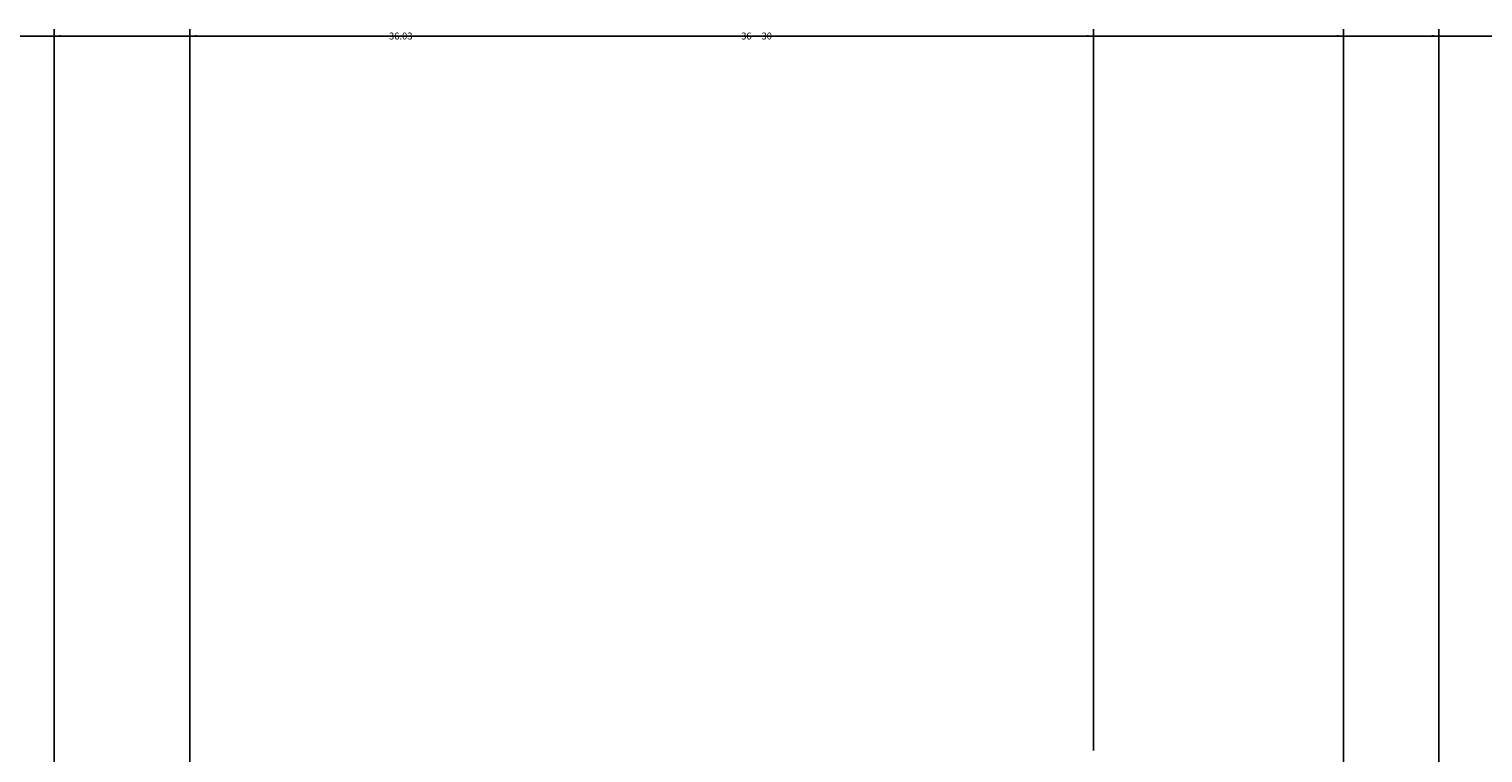
# Model space of a CAD drawing. Units: inches. Extents: x 2231 to 2461, y 2045 to 2455.
# Tile 77 of 95: x 2258 to 2296, y 2436 to 2455. Entities that reach past the tile are written whole.
import ezdxf

# ---------------------------------------------------------------- set-up
doc = ezdxf.new("R2010")
doc.units = ezdxf.units.IN
doc.layers.add('A-ANNO-DIMS', color=2, linetype='Continuous', lineweight=18)
doc.styles.get("Standard").update_dxf_attribs({"font": 'arial.ttf'})
doc.dimstyles.get("Standard").update_dxf_attribs({"dimtxt": 0.18, "dimasz": 0.18, "dimexe": 0.18, "dimexo": 0.0625, "dimgap": 0.09, "dimtad": 0, "dimtih": 1, "dimtoh": 1, "dimdec": 4, "dimzin": 0, "dimdsep": 46, "dimtxsty": 'Standard', "dimcen": 0.09, "dimadec": 0, "dimazin": 0, "dimtfac": 1, "dimtdec": 4, "dimtofl": 0, "dimtmove": 0, "dimatfit": 3, "dimfxl": 1, "dimtolj": 1, "dimtzin": 0, "dimarcsym": 0})

# ---------------------------------------------------------------- blocks, each defined once
blk = doc.blocks.new('*D35')
at = {"layer": 'A-ANNO-DIMS', "color": 0, "lineweight": -2, "transparency": 16777216}
for p, q in [((2258.794, 2426.895), (2258.794, 2454.645)), ((2258.974, 2454.465), (2313.513, 2454.465)), ((2368.614, 2454.465), (2314.074, 2454.465)), ((2368.794, 2426.895), (2368.794, 2454.645))]:
    blk.add_line(p, q, dxfattribs=at)
at = {"layer": 'A-ANNO-DIMS', "color": 0, "transparency": 16777216}
for points in [[(2258.974, 2454.495), (2258.974, 2454.435), (2258.794, 2454.465)], [(2368.614, 2454.495), (2368.614, 2454.435), (2368.794, 2454.465)]]:
    blk.add_solid(points, dxfattribs=at)
at = {"layer": 'Defpoints', "color": 0, "transparency": 16777216}
for p in [(2368.794, 2454.465), (2258.794, 2426.833), (2368.794, 2426.833)]:
    blk.add_point(p, dxfattribs=at)
at = {"layer": 'A-ANNO-DIMS', "color": 0, "transparency": 16777216, "insert": (2313.794, 2454.465), "char_height": 0.18, "attachment_point": 5}
blk.add_mtext('\\A1;110', dxfattribs=at)
blk = doc.blocks.new('*D47')
at = {"layer": 'A-ANNO-DIMS', "color": 0, "lineweight": -2, "transparency": 16777216}
for p, q in [((2258.794, 2182.895), (2258.794, 2454.645)), ((2258.974, 2454.465), (2276.575, 2454.465)), ((2294.614, 2454.465), (2277.012, 2454.465)), ((2294.794, 2182.895), (2294.794, 2454.645))]:
    blk.add_line(p, q, dxfattribs=at)
at = {"layer": 'A-ANNO-DIMS', "color": 0, "transparency": 16777216}
for points in [[(2258.974, 2454.495), (2258.974, 2454.435), (2258.794, 2454.465)], [(2294.614, 2454.495), (2294.614, 2454.435), (2294.794, 2454.465)]]:
    blk.add_solid(points, dxfattribs=at)
at = {"layer": 'Defpoints', "color": 0, "transparency": 16777216}
for p in [(2294.794, 2454.465), (2258.794, 2182.833), (2294.794, 2182.833)]:
    blk.add_point(p, dxfattribs=at)
at = {"layer": 'A-ANNO-DIMS', "color": 0, "transparency": 16777216, "insert": (2276.794, 2454.465), "char_height": 0.18, "attachment_point": 5}
blk.add_mtext('\\A1;36', dxfattribs=at)
blk = doc.blocks.new('*D55')
at = {"layer": 'A-ANNO-DIMS', "color": 0, "lineweight": -2, "transparency": 16777216}
for p, q in [((2249.794, 2435.895), (2249.794, 2454.645)), ((2249.974, 2454.465), (2267.413, 2454.465)), ((2285.64, 2454.465), (2268.2, 2454.465)), ((2285.82, 2435.895), (2285.82, 2454.645))]:
    blk.add_line(p, q, dxfattribs=at)
at = {"layer": 'A-ANNO-DIMS', "color": 0, "transparency": 16777216}
for points in [[(2249.974, 2454.495), (2249.974, 2454.435), (2249.794, 2454.465)], [(2285.64, 2454.495), (2285.64, 2454.435), (2285.82, 2454.465)]]:
    blk.add_solid(points, dxfattribs=at)
at = {"layer": 'Defpoints', "color": 0, "transparency": 16777216}
for p in [(2285.82, 2454.465), (2249.794, 2435.833), (2285.82, 2435.833)]:
    blk.add_point(p, dxfattribs=at)
at = {"layer": 'A-ANNO-DIMS', "color": 0, "transparency": 16777216, "insert": (2267.807, 2454.465), "char_height": 0.18, "attachment_point": 5}
blk.add_mtext('\\A1;36.03', dxfattribs=at)
blk = doc.blocks.new('*D62')
at = {"layer": 'A-ANNO-DIMS', "color": 0, "lineweight": -2, "transparency": 16777216}
for p, q in [((2262.321, 2255.176), (2262.321, 2454.645)), ((2262.501, 2454.465), (2277.102, 2454.465)), ((2292.141, 2454.465), (2277.539, 2454.465)), ((2292.321, 2253.176), (2292.321, 2454.645))]:
    blk.add_line(p, q, dxfattribs=at)
at = {"layer": 'A-ANNO-DIMS', "color": 0, "transparency": 16777216}
for points in [[(2262.501, 2454.495), (2262.501, 2454.435), (2262.321, 2454.465)], [(2292.141, 2454.495), (2292.141, 2454.435), (2292.321, 2454.465)]]:
    blk.add_solid(points, dxfattribs=at)
at = {"layer": 'Defpoints', "color": 0, "transparency": 16777216}
for p in [(2292.321, 2454.465), (2262.321, 2255.114), (2292.321, 2253.114)]:
    blk.add_point(p, dxfattribs=at)
at = {"layer": 'A-ANNO-DIMS', "color": 0, "transparency": 16777216, "insert": (2277.321, 2454.465), "char_height": 0.18, "attachment_point": 5}
blk.add_mtext('\\A1;30', dxfattribs=at)

msp = doc.modelspace()

# ---------------------------------------------------------------- dimensions: what is measured, and where the dimension line sits
at = {"layer": 'A-ANNO-DIMS'}
for base, p1, p2, override, picture, middle in [((2285.82, 2454.4653), (2249.7935, 2435.8328), (2285.82, 2435.8328), {"dimdec": 2, "dimlfac": 1, "dimrnd": 0, "dimzin": 0, "dimdsep": 46, "dimlunit": 2}, '*D55', (2267.8067, 2454.4653)), ((2368.7935, 2454.4653), (2258.7935, 2426.8328), (2368.7935, 2426.8328), {"dimdec": 0, "dimlfac": 1, "dimrnd": 0, "dimzin": 0, "dimdsep": 46, "dimlunit": 2}, '*D35', (2313.7935, 2454.4653)), ((2294.7935, 2454.4653), (2258.7935, 2182.8328), (2294.7935, 2182.8328), {"dimdec": 0, "dimlfac": 1, "dimrnd": 0, "dimzin": 0, "dimdsep": 46, "dimlunit": 2}, '*D47', (2276.7935, 2454.4653)), ((2292.3207, 2454.4653), (2262.3207, 2255.1137), (2292.3207, 2253.1137), {"dimdec": 0, "dimlfac": 1, "dimrnd": 0, "dimzin": 0, "dimdsep": 46, "dimlunit": 2}, '*D62', (2277.3207, 2454.4653))]:
    dim = msp.add_linear_dim(base=base, p1=p1, p2=p2, dimstyle='Standard', override=override, dxfattribs=at)
    dim.commit()
    dim.dimension.update_dxf_attribs({"geometry": picture, "text_midpoint": middle})

doc.saveas('drawing.dxf')
